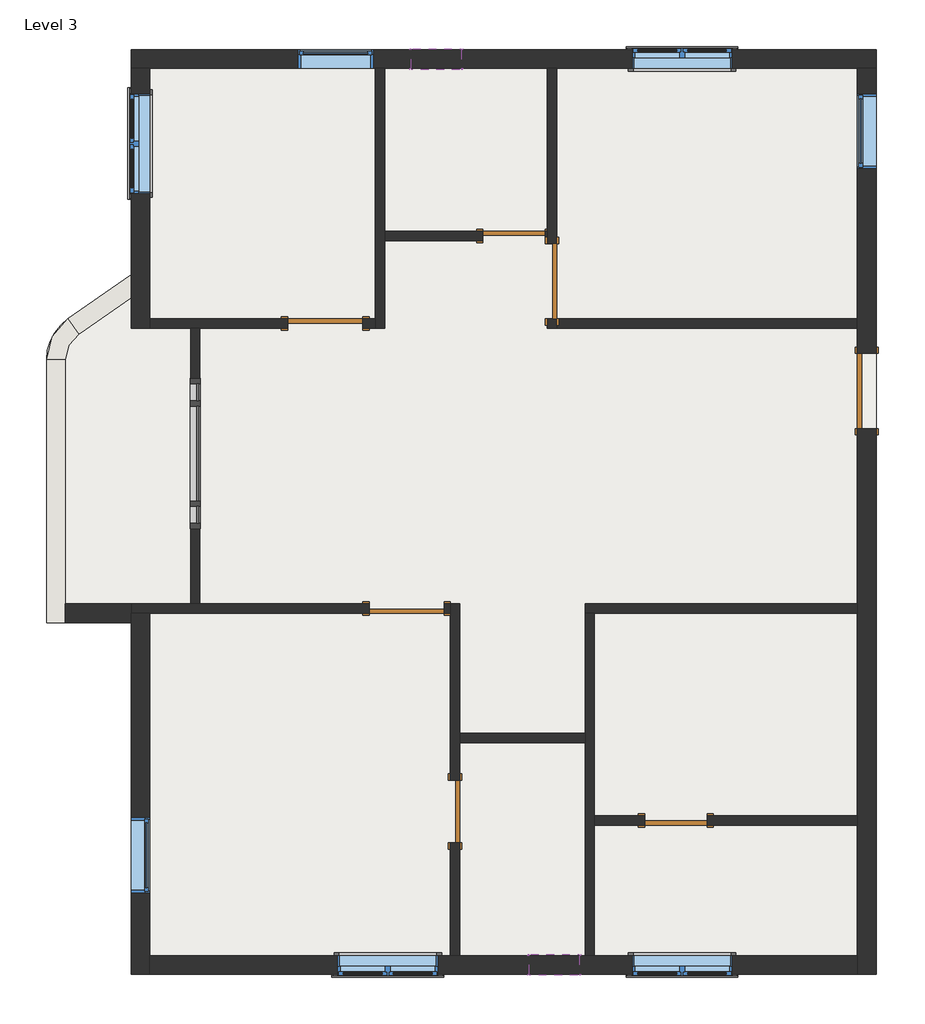
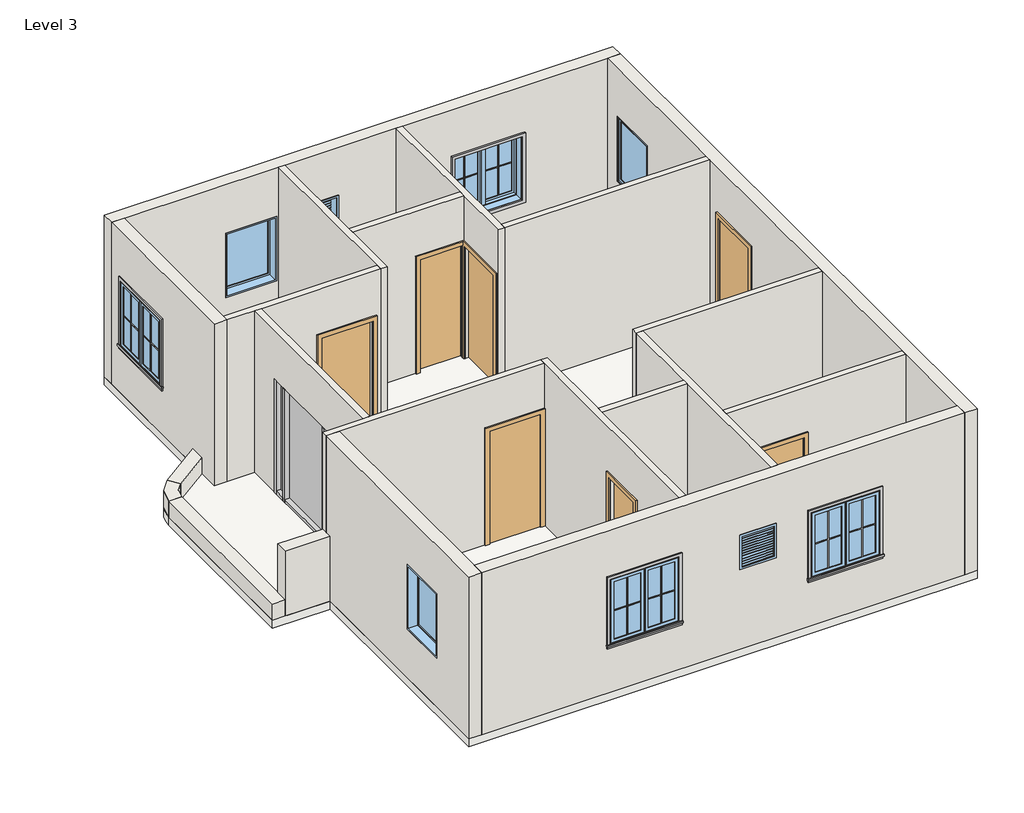
# One storey: 21 walls, 16 proxies, 9 windows, 7 doors, 7 members, 3 plates, 1 slab.
"""IFC4 building model written with IfcOpenShell, lengths in millimetres."""

from ifc_helpers import new_model, si_unit, point, frame, frame_2d, origin, place, context, project, spatial, polyline, circle_curve, trimmed, segment, composite_curve, outline, extrude, faceted_brep, transform, mapped, element, save
from components import muntin_pattern_2x2_muntin_pattern_2x2_4dfeb3f3, muntin_pattern_2x2_muntin_pattern_2x2_e852a7e4, trim_window_exterior_flat_with_sill_7cfdd449, trim_window_interior_flat_picture_frame_f1e0b15b, door_214872d5, door_78caadf7, door_e5f9f3c4, door_305aa2a5, door_0ca8825f, member_420b45ef, member_d7472725, member_7cbddb58, member_3374d9b6, system_panel_glazed_b82c55cd, system_panel_glazed_76d7ee11, window_c1f32544, window_af3140d2, window_f2d8fef0

model = new_model("IFC4")

# Units and contexts
model_context = context("Model", 3, world=origin())
ifc_project = project(units=[si_unit("LENGTHUNIT", "METRE", prefix="MILLI")], contexts=[model_context])

# Site, building, storey
site = spatial("IfcSite", under=ifc_project)
building = spatial("IfcBuilding", under=site)
storey = spatial("IfcBuildingStorey", under=building, Name="Level 3", Elevation=3200.4)

# Proxies
placement = place(None, origin())
muntin_pattern_2x2_muntin_pattern_2x2_shape = muntin_pattern_2x2_muntin_pattern_2x2_4dfeb3f3(model_context)
element("IfcBuildingElementProxy", 1, Name="Muntin Pattern_2x2 : Muntin Pattern_2x2", ObjectType="Muntin Pattern_2x2 : Muntin Pattern_2x2", at=placement, inside=storey, context=model_context, shape_type="MappedRepresentation", body=[
    mapped(muntin_pattern_2x2_muntin_pattern_2x2_shape, transform((-15529.7981107, 3990.1340181, 4184.65), x_axis=(0.0, 1.0, 0.0), y_axis=(-1.0, 0.0, 0.0), z_axis=(0.0, 0.0, 1.0))),
])
element("IfcBuildingElementProxy", 2, Name="Muntin Pattern_2x2 : Muntin Pattern_2x2", ObjectType="Muntin Pattern_2x2 : Muntin Pattern_2x2", at=placement, inside=storey, context=model_context, shape_type="MappedRepresentation", body=[
    mapped(muntin_pattern_2x2_muntin_pattern_2x2_shape, transform((-9136.9356107, 5426.8215181, 4184.65), x_axis=(1.0, 0.0, 0.0), y_axis=(0.0, 1.0, 0.0), z_axis=(0.0, 0.0, 1.0))),
])
element("IfcBuildingElementProxy", 3, Name="Muntin Pattern_2x2 : Muntin Pattern_2x2", ObjectType="Muntin Pattern_2x2 : Muntin Pattern_2x2", at=placement, inside=storey, context=model_context, shape_type="MappedRepresentation", body=[
    mapped(muntin_pattern_2x2_muntin_pattern_2x2_shape, transform((-12111.9106107, -5806.3284819, 4184.65), x_axis=(-1.0, 0.0, 0.0), y_axis=(0.0, -1.0, 0.0), z_axis=(0.0, 0.0, 1.0))),
])
element("IfcBuildingElementProxy", 4, Name="Muntin Pattern_2x2 : Muntin Pattern_2x2", ObjectType="Muntin Pattern_2x2 : Muntin Pattern_2x2", at=placement, inside=storey, context=model_context, shape_type="MappedRepresentation", body=[
    mapped(muntin_pattern_2x2_muntin_pattern_2x2_shape, transform((-8530.5106107, -5806.3284819, 4184.65), x_axis=(-1.0, 0.0, 0.0), y_axis=(0.0, -1.0, 0.0), z_axis=(0.0, 0.0, 1.0))),
])
muntin_pattern_2x2_muntin_pattern_2x2_2_shape = muntin_pattern_2x2_muntin_pattern_2x2_e852a7e4(model_context)
element("IfcBuildingElementProxy", 5, Name="Muntin Pattern_2x2 : Muntin Pattern_2x2", ObjectType="Muntin Pattern_2x2 : Muntin Pattern_2x2", at=placement, inside=storey, context=model_context, shape_type="MappedRepresentation", body=[
    mapped(muntin_pattern_2x2_muntin_pattern_2x2_2_shape, transform((-15529.7981107, 4596.5590181, 4184.65), x_axis=(0.0, -1.0, 0.0), y_axis=(1.0, 0.0, 0.0), z_axis=(0.0, 0.0, 1.0))),
])
element("IfcBuildingElementProxy", 6, Name="Muntin Pattern_2x2 : Muntin Pattern_2x2", ObjectType="Muntin Pattern_2x2 : Muntin Pattern_2x2", at=placement, inside=storey, context=model_context, shape_type="MappedRepresentation", body=[
    mapped(muntin_pattern_2x2_muntin_pattern_2x2_2_shape, transform((-8530.5106107, 5426.8215181, 4184.65), x_axis=(-1.0, 0.0, 0.0), y_axis=(0.0, -1.0, 0.0), z_axis=(0.0, 0.0, 1.0))),
])
element("IfcBuildingElementProxy", 7, Name="Muntin Pattern_2x2 : Muntin Pattern_2x2", ObjectType="Muntin Pattern_2x2 : Muntin Pattern_2x2", at=placement, inside=storey, context=model_context, shape_type="MappedRepresentation", body=[
    mapped(muntin_pattern_2x2_muntin_pattern_2x2_2_shape, transform((-12718.3356107, -5806.3284819, 4184.65), x_axis=(1.0, 0.0, 0.0), y_axis=(0.0, 1.0, 0.0), z_axis=(0.0, 0.0, 1.0))),
])
element("IfcBuildingElementProxy", 8, Name="Muntin Pattern_2x2 : Muntin Pattern_2x2", ObjectType="Muntin Pattern_2x2 : Muntin Pattern_2x2", at=placement, inside=storey, context=model_context, shape_type="MappedRepresentation", body=[
    mapped(muntin_pattern_2x2_muntin_pattern_2x2_2_shape, transform((-9136.9356107, -5806.3284819, 4184.65), x_axis=(1.0, 0.0, 0.0), y_axis=(0.0, 1.0, 0.0), z_axis=(0.0, 0.0, 1.0))),
])
trim_window_exterior_flat_with_sill_shape = trim_window_exterior_flat_with_sill_7cfdd449(model_context)
element("IfcBuildingElementProxy", 9, Name="Trim-Window-Exterior-Flat : with Sill", ObjectType="Trim-Window-Exterior-Flat : with Sill", at=placement, inside=storey, context=model_context, shape_type="MappedRepresentation", body=[
    mapped(trim_window_exterior_flat_with_sill_shape, transform((-15539.3231107, 4293.3465181, 5334.0), x_axis=(0.0, -1.0, 0.0), y_axis=(0.0, 0.0, 1.0), z_axis=(-1.0, 0.0, 0.0))),
])
element("IfcBuildingElementProxy", 10, Name="Trim-Window-Exterior-Flat : with Sill", ObjectType="Trim-Window-Exterior-Flat : with Sill", at=placement, inside=storey, context=model_context, shape_type="MappedRepresentation", body=[
    mapped(trim_window_exterior_flat_with_sill_shape, transform((-8833.7231107, 5436.3465181, 5334.0), x_axis=(-1.0, 0.0, 0.0), y_axis=(0.0, 0.0, 1.0), z_axis=(0.0, 1.0, 0.0))),
])
element("IfcBuildingElementProxy", 11, Name="Trim-Window-Exterior-Flat : with Sill", ObjectType="Trim-Window-Exterior-Flat : with Sill", at=placement, inside=storey, context=model_context, shape_type="MappedRepresentation", body=[
    mapped(trim_window_exterior_flat_with_sill_shape, transform((-12415.1231107, -5815.8534819, 5334.0), x_axis=(1.0, 0.0, 0.0), y_axis=(0.0, 0.0, 1.0), z_axis=(0.0, -1.0, 0.0))),
])
element("IfcBuildingElementProxy", 12, Name="Trim-Window-Exterior-Flat : with Sill", ObjectType="Trim-Window-Exterior-Flat : with Sill", at=placement, inside=storey, context=model_context, shape_type="MappedRepresentation", body=[
    mapped(trim_window_exterior_flat_with_sill_shape, transform((-8833.7231107, -5815.8534819, 5334.0), x_axis=(1.0, 0.0, 0.0), y_axis=(0.0, 0.0, 1.0), z_axis=(0.0, -1.0, 0.0))),
])
trim_window_interior_flat_picture_frame_shape = trim_window_interior_flat_picture_frame_f1e0b15b(model_context)
element("IfcBuildingElementProxy", 13, Name="Trim-Window-Interior-Flat : Picture Frame", ObjectType="Trim-Window-Interior-Flat : Picture Frame", at=placement, inside=storey, context=model_context, shape_type="MappedRepresentation", body=[
    mapped(trim_window_interior_flat_picture_frame_shape, transform((-15310.7231107, 4293.3465181, 5334.0), x_axis=(0.0, 1.0, 0.0), y_axis=(0.0, 0.0, 1.0), z_axis=(1.0, 0.0, 0.0))),
])
element("IfcBuildingElementProxy", 14, Name="Trim-Window-Interior-Flat : Picture Frame", ObjectType="Trim-Window-Interior-Flat : Picture Frame", at=placement, inside=storey, context=model_context, shape_type="MappedRepresentation", body=[
    mapped(trim_window_interior_flat_picture_frame_shape, transform((-8833.7231107, 5207.7465181, 5334.0), x_axis=(1.0, 0.0, 0.0), y_axis=(0.0, 0.0, 1.0), z_axis=(0.0, -1.0, 0.0))),
])
element("IfcBuildingElementProxy", 15, Name="Trim-Window-Interior-Flat : Picture Frame", ObjectType="Trim-Window-Interior-Flat : Picture Frame", at=placement, inside=storey, context=model_context, shape_type="MappedRepresentation", body=[
    mapped(trim_window_interior_flat_picture_frame_shape, transform((-12415.1231107, -5587.2534819, 5334.0), x_axis=(-1.0, 0.0, 0.0), y_axis=(0.0, 0.0, 1.0), z_axis=(0.0, 1.0, 0.0))),
])
element("IfcBuildingElementProxy", 16, Name="Trim-Window-Interior-Flat : Picture Frame", ObjectType="Trim-Window-Interior-Flat : Picture Frame", at=placement, inside=storey, context=model_context, shape_type="MappedRepresentation", body=[
    mapped(trim_window_interior_flat_picture_frame_shape, transform((-8833.7231107, -5587.2534819, 5334.0), x_axis=(-1.0, 0.0, 0.0), y_axis=(0.0, 0.0, 1.0), z_axis=(0.0, 1.0, 0.0))),
])

# Doors
door_shape = door_214872d5(model_context)
element("IfcDoor", 17, ObjectType="Single-Flush : 2'6\" X 7'", at=placement, inside=storey, context=model_context, shape_type="MappedRepresentation", body=[
    mapped(door_shape, transform((-10878.4231107, 3169.3965181, 3200.4), x_axis=(1.0, 0.0, 0.0), y_axis=(0.0, 1.0, 0.0), z_axis=(0.0, 0.0, 1.0))),
])
element("IfcDoor", 18, ObjectType="Single-Flush : 2'6\" X 7'", at=placement, inside=storey, context=model_context, shape_type="MappedRepresentation", body=[
    mapped(door_shape, transform((-8909.9231107, -3942.6034819, 3200.4), x_axis=(-1.0, 0.0, 0.0), y_axis=(0.0, -1.0, 0.0), z_axis=(0.0, 0.0, 1.0))),
])
door_2_shape = door_78caadf7(model_context)
element("IfcDoor", 19, ObjectType="Single-Flush : 2'6\" X 7'", at=placement, inside=storey, context=model_context, shape_type="MappedRepresentation", body=[
    mapped(door_2_shape, transform((-11595.9731107, -3834.6534819, 3200.4), x_axis=(0.0, 1.0, 0.0), y_axis=(-1.0, 0.0, 0.0), z_axis=(0.0, 0.0, 1.0))),
])
door_3_shape = door_e5f9f3c4(model_context)
element("IfcDoor", 20, ObjectType="Single-Flush : 36\" x 84\"", at=placement, inside=storey, context=model_context, shape_type="MappedRepresentation", body=[
    mapped(door_3_shape, transform((-13177.1231107, 2102.5965181, 3200.4), x_axis=(1.0, 0.0, 0.0), y_axis=(0.0, 1.0, 0.0), z_axis=(0.0, 0.0, 1.0))),
])
element("IfcDoor", 21, ObjectType="Single-Flush : 36\" x 84\"", at=placement, inside=storey, context=model_context, shape_type="MappedRepresentation", body=[
    mapped(door_3_shape, transform((-10414.8731107, 2618.6439204, 3200.4), x_axis=(0.0, -1.0, 0.0), y_axis=(1.0, 0.0, 0.0), z_axis=(0.0, 0.0, 1.0))),
])
door_4_shape = door_305aa2a5(model_context)
element("IfcDoor", 22, ObjectType="Single-Flush : 36\" x 84\"", at=placement, inside=storey, context=model_context, shape_type="MappedRepresentation", body=[
    mapped(door_4_shape, transform((-12186.5231107, -1364.5034819, 3200.4), x_axis=(1.0, 0.0, 0.0), y_axis=(0.0, 1.0, 0.0), z_axis=(0.0, 0.0, 1.0))),
])
door_5_shape = door_0ca8825f(model_context)
element("IfcDoor", 23, ObjectType="Single-Flush : 36\" x 84\"", at=placement, inside=storey, context=model_context, shape_type="MappedRepresentation", body=[
    mapped(door_5_shape, transform((-6585.8231107, 1283.4465181, 3200.4), x_axis=(0.0, 1.0, 0.0), y_axis=(-1.0, 0.0, 0.0), z_axis=(0.0, 0.0, 1.0))),
])

# Members
member_shape = member_420b45ef(model_context)
element("IfcMember", 24, ObjectType="Rectangular Mullion : 2.5\" x 5\" rectangular", at=placement, inside=storey, context=model_context, shape_type="MappedRepresentation", body=[
    mapped(member_shape, transform((-14758.2731107, 1372.3465181, 3200.4), x_axis=(0.0, 0.0, -1.0), y_axis=(-1.0, 0.0, 0.0), z_axis=(0.0, 1.0, 0.0))),
])
element("IfcMember", 25, ObjectType="Rectangular Mullion : 2.5\" x 5\" rectangular", at=placement, inside=storey, context=model_context, shape_type="MappedRepresentation", body=[
    mapped(member_shape, transform((-14758.2731107, -119.9034819, 3200.4), x_axis=(0.0, 0.0, -1.0), y_axis=(-1.0, 0.0, 0.0), z_axis=(0.0, 1.0, 0.0))),
])
member_2_shape = member_d7472725(model_context)
element("IfcMember", 26, ObjectType="Rectangular Mullion : 2.5\" x 5\" rectangular", at=placement, inside=storey, context=model_context, shape_type="MappedRepresentation", body=[
    mapped(member_2_shape, transform((-14758.2731107, 1099.2965181, 3200.4), x_axis=(0.0, 0.0, -1.0), y_axis=(-1.0, 0.0, 0.0), z_axis=(0.0, 1.0, 0.0))),
])
member_3_shape = member_7cbddb58(model_context)
element("IfcMember", 27, ObjectType="Rectangular Mullion : 2.5\" x 5\" rectangular", at=placement, inside=storey, context=model_context, shape_type="MappedRepresentation", body=[
    mapped(member_3_shape, transform((-14758.2731107, 1131.0465181, 3200.4), x_axis=(0.0, -1.0, 0.0), y_axis=(-1.0, 0.0, 0.0), z_axis=(0.0, 0.0, -1.0))),
])
element("IfcMember", 28, ObjectType="Rectangular Mullion : 2.5\" x 5\" rectangular", at=placement, inside=storey, context=model_context, shape_type="MappedRepresentation", body=[
    mapped(member_3_shape, transform((-14758.2731107, -88.1534819, 3200.4), x_axis=(0.0, -1.0, 0.0), y_axis=(-1.0, 0.0, 0.0), z_axis=(0.0, 0.0, -1.0))),
])
member_4_shape = member_3374d9b6(model_context)
element("IfcMember", 29, ObjectType="Rectangular Mullion : 2.5\" x 5\" rectangular", at=placement, inside=storey, context=model_context, shape_type="MappedRepresentation", body=[
    mapped(member_4_shape, transform((-14758.2731107, 1435.8465181, 5334.0), x_axis=(0.0, 1.0, 0.0), y_axis=(-1.0, 0.0, 0.0), z_axis=(0.0, 0.0, 1.0))),
])
element("IfcMember", 30, ObjectType="Rectangular Mullion : 2.5\" x 5\" rectangular", at=placement, inside=storey, context=model_context, shape_type="MappedRepresentation", body=[
    mapped(member_4_shape, transform((-14758.2731107, -392.9534819, 3200.4), x_axis=(0.0, -1.0, 0.0), y_axis=(-1.0, 0.0, 0.0), z_axis=(0.0, 0.0, -1.0))),
])

# Plates
system_panel_glazed_shape = system_panel_glazed_b82c55cd(model_context)
element("IfcPlate", 31, ObjectType="System Panel : Glazed", at=placement, inside=storey, context=model_context, shape_type="MappedRepresentation", body=[
    mapped(system_panel_glazed_shape, transform((-14758.2731107, 1267.5715181, 3263.9), x_axis=(0.0, -1.0, 0.0), y_axis=(1.0, 0.0, 0.0), z_axis=(0.0, 0.0, 1.0))),
])
element("IfcPlate", 32, ObjectType="System Panel : Glazed", at=placement, inside=storey, context=model_context, shape_type="MappedRepresentation", body=[
    mapped(system_panel_glazed_shape, transform((-14758.2731107, -224.6784819, 3263.9), x_axis=(0.0, -1.0, 0.0), y_axis=(1.0, 0.0, 0.0), z_axis=(0.0, 0.0, 1.0))),
])
system_panel_glazed_2_shape = system_panel_glazed_76d7ee11(model_context)
element("IfcPlate", 33, ObjectType="System Panel : Glazed", at=placement, inside=storey, context=model_context, shape_type="MappedRepresentation", body=[
    mapped(system_panel_glazed_2_shape, transform((-14758.2731107, 521.4465181, 3263.9), x_axis=(0.0, -1.0, 0.0), y_axis=(1.0, 0.0, 0.0), z_axis=(0.0, 0.0, 1.0))),
])

# Slab
element("IfcSlab", 34, ObjectType="6\"", at=placement, inside=storey, context=model_context, shape_type="SweptSolid", body=[
    extrude(outline(composite_curve([segment(polyline([(-6471.5231107, 5436.3465181), (-6471.5231107, -5815.8534819), (-15539.3231107, -5815.8534819), (-15539.3231107, -1535.9534819), (-16568.0231107, -1535.9534819), (-16568.0231107, 1661.5585867)]), True, "CONTINUOUS"), segment(trimmed(circle_curve(frame_2d((-15958.4231107, 1661.5585867)), 609.6), [point((-16568.0231107, 1661.5585867))], [point((-16308.0753063, 2160.9136729))], False, "CARTESIAN"), True, "CONTINUOUS"), segment(polyline([(-16308.0753063, 2160.9136729), (-15539.3231107, 2699.1997553), (-15539.3231107, 5436.3465181), (-6471.5231107, 5436.3465181)]), True, "CONTINUOUS")], self_intersect=False)), frame((0.0, 0.0, 3048.0), z_axis=(0.0, 0.0, 1.0), x_axis=(1.0, 0.0, 0.0)), (0.0, 0.0, 1.0), 152.4),
])

# Walls
element("IfcWall", 35, ObjectType="4.5\"", at=placement, inside=storey, context=model_context, shape_type="Brep", body=[
    faceted_brep([(-12567.5231107, 5207.7465181, 3200.4), (-12567.5231107, 2159.7465181, 3200.4), (-12567.5231107, 2045.4465181, 3200.4), (-12567.5231107, 2045.4465181, 6248.4), (-12567.5231107, 2159.7465181, 6248.4), (-12567.5231107, 5207.7465181, 6248.4), (-12453.2231107, 5207.7465181, 3200.4), (-12453.2231107, 5207.7465181, 6248.4), (-12453.2231107, 3226.5465181, 6248.4), (-12453.2231107, 3112.2465181, 6248.4), (-12453.2231107, 2045.4465181, 6248.4), (-12453.2231107, 2045.4465181, 3200.4), (-12453.2231107, 3112.2465181, 3200.4), (-12453.2231107, 3226.5465181, 3200.4)], [[[0, 1, 2, 3, 4, 5]], [[6, 7, 8, 9, 10, 11, 12, 13]], [[2, 1, 0, 6, 13, 12, 11]], [[5, 4, 3, 10, 9, 8, 7]], [[0, 5, 7, 6]], [[3, 2, 11, 10]]]),
])
element("IfcWall", 36, ObjectType="4.5\"", at=placement, inside=storey, context=model_context, shape_type="Brep", body=[
    faceted_brep([(-12719.9231107, 2045.4465181, 5334.0), (-12719.9231107, 2045.4465181, 3200.4), (-12567.5231107, 2045.4465181, 3200.4), (-12567.5231107, 2045.4465181, 6248.4), (-14701.1231107, 2045.4465181, 6248.4), (-14815.4231107, 2045.4465181, 6248.4), (-15310.7231107, 2045.4465181, 6248.4), (-15310.7231107, 2045.4465181, 3200.4), (-14815.4231107, 2045.4465181, 3200.4), (-14701.1231107, 2045.4465181, 3200.4), (-13634.3231107, 2045.4465181, 3200.4), (-13634.3231107, 2045.4465181, 5334.0), (-12567.5231107, 2159.7465181, 3200.4), (-12719.9231107, 2159.7465181, 3200.4), (-12719.9231107, 2159.7465181, 5334.0), (-13634.3231107, 2159.7465181, 5334.0), (-13634.3231107, 2159.7465181, 3200.4), (-15310.7231107, 2159.7465181, 3200.4), (-15310.7231107, 2159.7465181, 6248.4), (-12567.5231107, 2159.7465181, 6248.4)], [[[0, 1, 2, 3, 4, 5, 6, 7, 8, 9, 10, 11]], [[12, 13, 14, 15, 16, 17, 18, 19]], [[2, 1, 13, 12]], [[10, 9, 8, 7, 17, 16]], [[6, 5, 4, 3, 19, 18]], [[3, 2, 12, 19]], [[7, 6, 18, 17]], [[14, 13, 1, 0]], [[15, 14, 0, 11]], [[16, 15, 11, 10]]]),
])
element("IfcWall", 37, ObjectType="4.5\"", at=placement, inside=storey, context=model_context, shape_type="Brep", body=[
    faceted_brep([(-10472.0231107, 2161.4439204, 5334.0), (-10472.0231107, 2161.4439204, 3200.4), (-10472.0231107, 2045.4465181, 3200.4), (-10472.0231107, 2045.4465181, 6248.4), (-10472.0231107, 3112.2465181, 6248.4), (-10472.0231107, 3226.5465181, 6248.4), (-10472.0231107, 5207.7465181, 6248.4), (-10472.0231107, 5207.7465181, 3200.4), (-10472.0231107, 3226.5465181, 3200.4), (-10472.0231107, 3112.2465181, 3200.4), (-10472.0231107, 3075.8439204, 3200.4), (-10472.0231107, 3075.8439204, 5334.0), (-10357.7231107, 2045.4465181, 3200.4), (-10357.7231107, 2159.7465181, 3200.4), (-10357.7231107, 2161.4439204, 3200.4), (-10357.7231107, 2161.4439204, 5334.0), (-10357.7231107, 3075.8439204, 5334.0), (-10357.7231107, 3075.8439204, 3200.4), (-10357.7231107, 5207.7465181, 3200.4), (-10357.7231107, 5207.7465181, 6248.4), (-10357.7231107, 2159.7465181, 6248.4), (-10357.7231107, 2045.4465181, 6248.4)], [[[0, 1, 2, 3, 4, 5, 6, 7, 8, 9, 10, 11]], [[12, 13, 14, 15, 16, 17, 18, 19, 20, 21]], [[2, 1, 14, 13, 12]], [[10, 9, 8, 7, 18, 17]], [[6, 5, 4, 3, 21, 20, 19]], [[7, 6, 19, 18]], [[3, 2, 12, 21]], [[15, 14, 1, 0]], [[16, 15, 0, 11]], [[17, 16, 11, 10]]]),
])
element("IfcWall", 38, ObjectType="4.5\"", at=placement, inside=storey, context=model_context, shape_type="SweptSolid", body=[
    extrude(outline(polyline([(5334.0, -10497.4231107), (3200.4, -10497.4231107), (3200.4, -10472.0231107), (6248.4, -10472.0231107), (6248.4, -12453.2231107), (3200.4, -12453.2231107), (3200.4, -11259.4231107), (5334.0, -11259.4231107), (5334.0, -10497.4231107)])), frame((0.0, 3112.2465181, 0.0), z_axis=(0.0, 1.0, 0.0), x_axis=(0.0, 0.0, 1.0)), (0.0, 0.0, 1.0), 114.3),
])
element("IfcWall", 39, ObjectType="4.5\"", at=placement, inside=storey, context=model_context, shape_type="SweptSolid", body=[
    extrude(outline(polyline([(-10357.7231107, 2159.7465181), (-6700.1231107, 2159.7465181), (-6700.1231107, 2045.4465181), (-10357.7231107, 2045.4465181), (-10357.7231107, 2159.7465181)])), frame((0.0, 0.0, 3200.4), z_axis=(0.0, 0.0, 1.0), x_axis=(1.0, 0.0, 0.0)), (0.0, 0.0, 1.0), 3048.0),
])
element("IfcWall", 40, ObjectType="4.5\"", at=placement, inside=storey, context=model_context, shape_type="Brep", body=[
    faceted_brep([(-6700.1231107, -1307.3534819, 3200.4), (-10014.8231107, -1307.3534819, 3200.4), (-10014.8231107, -1307.3534819, 6248.4), (-6700.1231107, -1307.3534819, 6248.4), (-6700.1231107, -1421.6534819, 3200.4), (-6700.1231107, -1421.6534819, 6248.4), (-9900.5231107, -1421.6534819, 6248.4), (-10014.8231107, -1421.6534819, 6248.4), (-10014.8231107, -1421.6534819, 3200.4), (-9900.5231107, -1421.6534819, 3200.4)], [[[0, 1, 2, 3]], [[4, 5, 6, 7, 8, 9]], [[1, 0, 4, 9, 8]], [[3, 2, 7, 6, 5]], [[0, 3, 5, 4]], [[2, 1, 8, 7]]]),
])
element("IfcWall", 41, ObjectType="4.5\"", at=placement, inside=storey, context=model_context, shape_type="SweptSolid", body=[
    extrude(outline(polyline([(3200.4, -9900.5231107), (3200.4, -9290.9231107), (5334.0, -9290.9231107), (5334.0, -8528.9231107), (3200.4, -8528.9231107), (3200.4, -6700.1231107), (6248.4, -6700.1231107), (6248.4, -9900.5231107), (3200.4, -9900.5231107)])), frame((0.0, -3999.7534819, 0.0), z_axis=(0.0, 1.0, 0.0), x_axis=(0.0, 0.0, 1.0)), (0.0, 0.0, 1.0), 114.3),
])
element("IfcWall", 42, ObjectType="4.5\"", at=placement, inside=storey, context=model_context, shape_type="Brep", body=[
    faceted_brep([(-9900.5231107, -5587.2534819, 3200.4), (-9900.5231107, -3999.7534819, 3200.4), (-9900.5231107, -3885.4534819, 3200.4), (-9900.5231107, -1421.6534819, 3200.4), (-9900.5231107, -1421.6534819, 6248.4), (-9900.5231107, -3885.4534819, 6248.4), (-9900.5231107, -3999.7534819, 6248.4), (-9900.5231107, -5587.2534819, 6248.4), (-10014.8231107, -5587.2534819, 3200.4), (-10014.8231107, -5587.2534819, 6248.4), (-10014.8231107, -2996.4534819, 6248.4), (-10014.8231107, -2882.1534819, 6248.4), (-10014.8231107, -1421.6534819, 6248.4), (-10014.8231107, -1421.6534819, 3200.4), (-10014.8231107, -2882.1534819, 3200.4), (-10014.8231107, -2996.4534819, 3200.4)], [[[0, 1, 2, 3, 4, 5, 6, 7]], [[8, 9, 10, 11, 12, 13, 14, 15]], [[3, 2, 1, 0, 8, 15, 14, 13]], [[7, 6, 5, 4, 12, 11, 10, 9]], [[0, 7, 9, 8]], [[4, 3, 13, 12]]]),
])
element("IfcWall", 43, ObjectType="4.5\"", at=placement, inside=storey, context=model_context, shape_type="Brep", body=[
    faceted_brep([(-11538.8231107, -3453.6534819, 5334.0), (-11538.8231107, -3453.6534819, 3200.4), (-11538.8231107, -2996.4534819, 3200.4), (-11538.8231107, -2882.1534819, 3200.4), (-11538.8231107, -1307.3534819, 3200.4), (-11538.8231107, -1307.3534819, 6248.4), (-11538.8231107, -2882.1534819, 6248.4), (-11538.8231107, -2996.4534819, 6248.4), (-11538.8231107, -5587.2534819, 6248.4), (-11538.8231107, -5587.2534819, 3200.4), (-11538.8231107, -4215.6534819, 3200.4), (-11538.8231107, -4215.6534819, 5334.0), (-11653.1231107, -1307.3534819, 3200.4), (-11653.1231107, -1421.6534819, 3200.4), (-11653.1231107, -3453.6534819, 3200.4), (-11653.1231107, -3453.6534819, 5334.0), (-11653.1231107, -4215.6534819, 5334.0), (-11653.1231107, -4215.6534819, 3200.4), (-11653.1231107, -5587.2534819, 3200.4), (-11653.1231107, -5587.2534819, 6248.4), (-11653.1231107, -1421.6534819, 6248.4), (-11653.1231107, -1307.3534819, 6248.4)], [[[0, 1, 2, 3, 4, 5, 6, 7, 8, 9, 10, 11]], [[12, 13, 14, 15, 16, 17, 18, 19, 20, 21]], [[10, 9, 18, 17]], [[4, 3, 2, 1, 14, 13, 12]], [[8, 7, 6, 5, 21, 20, 19]], [[9, 8, 19, 18]], [[5, 4, 12, 21]], [[15, 14, 1, 0]], [[16, 15, 0, 11]], [[17, 16, 11, 10]]]),
])
element("IfcWall", 44, ObjectType="4.5\"", at=placement, inside=storey, context=model_context, shape_type="SweptSolid", body=[
    extrude(outline(polyline([(-10014.8231107, -2996.4534819), (-11538.8231107, -2996.4534819), (-11538.8231107, -2882.1534819), (-10014.8231107, -2882.1534819), (-10014.8231107, -2996.4534819)])), frame((0.0, 0.0, 3200.4), z_axis=(0.0, 0.0, 1.0), x_axis=(1.0, 0.0, 0.0)), (0.0, 0.0, 1.0), 3048.0),
])
element("IfcWall", 45, ObjectType="4.5\"", at=placement, inside=storey, context=model_context, shape_type="Brep", body=[
    faceted_brep([(-11653.1231107, -1307.3534819, 3200.4), (-11729.3231107, -1307.3534819, 3200.4), (-11729.3231107, -1307.3534819, 5334.0), (-12643.7231107, -1307.3534819, 5334.0), (-12643.7231107, -1307.3534819, 3200.4), (-14701.1231107, -1307.3534819, 3200.4), (-14815.4231107, -1307.3534819, 3200.4), (-15539.3231107, -1307.3534819, 3200.4), (-15539.3231107, -1307.3534819, 4419.6), (-15539.3231107, -1307.3534819, 6248.4), (-14815.4231107, -1307.3534819, 6248.4), (-14701.1231107, -1307.3534819, 6248.4), (-11653.1231107, -1307.3534819, 6248.4), (-11729.3231107, -1421.6534819, 5334.0), (-11729.3231107, -1421.6534819, 3200.4), (-11653.1231107, -1421.6534819, 3200.4), (-11653.1231107, -1421.6534819, 6248.4), (-15310.7231107, -1421.6534819, 6248.4), (-15539.3231107, -1421.6534819, 6248.4), (-15539.3231107, -1421.6534819, 3200.4), (-15310.7231107, -1421.6534819, 3200.4), (-12643.7231107, -1421.6534819, 3200.4), (-12643.7231107, -1421.6534819, 5334.0)], [[[0, 1, 2, 3, 4, 5, 6, 7, 8, 9, 10, 11, 12]], [[13, 14, 15, 16, 17, 18, 19, 20, 21, 22]], [[15, 14, 1, 0]], [[21, 20, 19, 7, 6, 5, 4]], [[12, 11, 10, 9, 18, 17, 16]], [[0, 12, 16, 15]], [[2, 1, 14, 13]], [[3, 2, 13, 22]], [[4, 3, 22, 21]], [[7, 19, 18, 9, 8]]]),
])
element("IfcWall", 46, ObjectType="4.5\"", at=placement, inside=storey, context=model_context, shape_type="SweptSolid", body=[
    extrude(outline(polyline([(-1307.3534819, 6248.4), (2045.4465181, 6248.4), (2045.4465181, 3200.4), (1435.8465181, 3200.4), (1435.8465181, 5334.0), (-392.9534819, 5334.0), (-392.9534819, 3200.4), (-1307.3534819, 3200.4), (-1307.3534819, 6248.4)])), frame((-14815.4231107, 0.0, 0.0), z_axis=(1.0, 0.0, 0.0), x_axis=(0.0, 1.0, 0.0)), (0.0, 0.0, 1.0), 114.3),
])
element("IfcWall", 47, ObjectType="9\"", at=placement, inside=storey, context=model_context, shape_type="Brep", body=[
    faceted_brep([(-15539.3231107, 5207.7465181, 3200.4), (-15310.7231107, 5207.7465181, 3200.4), (-12567.5231107, 5207.7465181, 3200.4), (-12453.2231107, 5207.7465181, 3200.4), (-10472.0231107, 5207.7465181, 3200.4), (-10357.7231107, 5207.7465181, 3200.4), (-6700.1231107, 5207.7465181, 3200.4), (-6471.5231107, 5207.7465181, 3200.4), (-6471.5231107, 5207.7465181, 6248.4), (-6700.1231107, 5207.7465181, 6248.4), (-10357.7231107, 5207.7465181, 6248.4), (-10472.0231107, 5207.7465181, 6248.4), (-12453.2231107, 5207.7465181, 6248.4), (-12567.5231107, 5207.7465181, 6248.4), (-15310.7231107, 5207.7465181, 6248.4), (-15539.3231107, 5207.7465181, 6248.4), (-12129.3731107, 5207.7465181, 5334.0), (-11519.7731107, 5207.7465181, 5334.0), (-11519.7731107, 5207.7465181, 4724.4), (-12129.3731107, 5207.7465181, 4724.4), (-8224.1231107, 5207.7465181, 5334.0), (-8224.1231107, 5207.7465181, 4114.8), (-9443.3231107, 5207.7465181, 4114.8), (-9443.3231107, 5207.7465181, 5334.0), (-12592.9231107, 5207.7465181, 5334.0), (-12592.9231107, 5207.7465181, 4114.8), (-13507.3231107, 5207.7465181, 4114.8), (-13507.3231107, 5207.7465181, 5334.0), (-15539.3231107, 5436.3465181, 3200.4), (-15539.3231107, 5436.3465181, 6248.4), (-6471.5231107, 5436.3465181, 6248.4), (-6471.5231107, 5436.3465181, 3200.4), (-12129.3731107, 5436.3465181, 5334.0), (-12129.3731107, 5436.3465181, 4724.4), (-11519.7731107, 5436.3465181, 4724.4), (-11519.7731107, 5436.3465181, 5334.0), (-8224.1231107, 5436.3465181, 5334.0), (-9443.3231107, 5436.3465181, 5334.0), (-9443.3231107, 5436.3465181, 4114.8), (-8224.1231107, 5436.3465181, 4114.8), (-12592.9231107, 5436.3465181, 5334.0), (-13507.3231107, 5436.3465181, 5334.0), (-13507.3231107, 5436.3465181, 4114.8), (-12592.9231107, 5436.3465181, 4114.8)], [[[0, 1, 2, 3, 4, 5, 6, 7, 8, 9, 10, 11, 12, 13, 14, 15], [16, 17, 18, 19], [20, 21, 22, 23], [24, 25, 26, 27]], [[28, 29, 30, 31], [32, 33, 34, 35], [36, 37, 38, 39], [40, 41, 42, 43]], [[7, 6, 5, 4, 3, 2, 1, 0, 28, 31]], [[15, 14, 13, 12, 11, 10, 9, 8, 30, 29]], [[0, 15, 29, 28]], [[8, 7, 31, 30]], [[33, 32, 16, 19]], [[34, 33, 19, 18]], [[35, 34, 18, 17]], [[32, 35, 17, 16]], [[21, 20, 36, 39]], [[22, 21, 39, 38]], [[23, 22, 38, 37]], [[20, 23, 37, 36]], [[25, 24, 40, 43]], [[26, 25, 43, 42]], [[27, 26, 42, 41]], [[24, 27, 41, 40]]]),
])
element("IfcWall", 48, ObjectType="9\"", at=placement, inside=storey, context=model_context, shape_type="Brep", body=[
    faceted_brep([(-15539.3231107, 5207.7465181, 3200.4), (-15539.3231107, 2699.1997553, 3200.4), (-15539.3231107, 2420.1306843, 3200.4), (-15539.3231107, 2045.4465181, 3200.4), (-15539.3231107, 2045.4465181, 6248.4), (-15539.3231107, 5207.7465181, 6248.4), (-15539.3231107, 4902.9465181, 5334.0), (-15539.3231107, 3683.7465181, 5334.0), (-15539.3231107, 3683.7465181, 4114.8), (-15539.3231107, 4902.9465181, 4114.8), (-15310.7231107, 5207.7465181, 3200.4), (-15310.7231107, 5207.7465181, 6248.4), (-15310.7231107, 2159.7465181, 6248.4), (-15310.7231107, 2045.4465181, 6248.4), (-15310.7231107, 2045.4465181, 3200.4), (-15310.7231107, 2159.7465181, 3200.4), (-15310.7231107, 4902.9465181, 5334.0), (-15310.7231107, 4902.9465181, 4114.8), (-15310.7231107, 3683.7465181, 4114.8), (-15310.7231107, 3683.7465181, 5334.0)], [[[0, 1, 2, 3, 4, 5], [6, 7, 8, 9]], [[10, 11, 12, 13, 14, 15], [16, 17, 18, 19]], [[3, 2, 1, 0, 10, 15, 14]], [[5, 4, 13, 12, 11]], [[0, 5, 11, 10]], [[4, 3, 14, 13]], [[17, 16, 6, 9]], [[18, 17, 9, 8]], [[19, 18, 8, 7]], [[16, 19, 7, 6]]]),
])
element("IfcWall", 49, ObjectType="9\"", at=placement, inside=storey, context=model_context, shape_type="Brep", body=[
    faceted_brep([(-6700.1231107, 5207.7465181, 3200.4), (-6700.1231107, 2159.7465181, 3200.4), (-6700.1231107, 2045.4465181, 3200.4), (-6700.1231107, 1740.6465181, 3200.4), (-6700.1231107, 1740.6465181, 5334.0), (-6700.1231107, 826.2465181, 5334.0), (-6700.1231107, 826.2465181, 3200.4), (-6700.1231107, -1307.3534819, 3200.4), (-6700.1231107, -1421.6534819, 3200.4), (-6700.1231107, -3885.4534819, 3200.4), (-6700.1231107, -3999.7534819, 3200.4), (-6700.1231107, -5587.2534819, 3200.4), (-6700.1231107, -5815.8534819, 3200.4), (-6700.1231107, -5815.8534819, 6248.4), (-6700.1231107, -5587.2534819, 6248.4), (-6700.1231107, -3999.7534819, 6248.4), (-6700.1231107, -3885.4534819, 6248.4), (-6700.1231107, -1421.6534819, 6248.4), (-6700.1231107, -1307.3534819, 6248.4), (-6700.1231107, 2045.4465181, 6248.4), (-6700.1231107, 2159.7465181, 6248.4), (-6700.1231107, 5207.7465181, 6248.4), (-6700.1231107, 4902.9465181, 5334.0), (-6700.1231107, 3988.5465181, 5334.0), (-6700.1231107, 3988.5465181, 4114.8), (-6700.1231107, 4902.9465181, 4114.8), (-6471.5231107, 1740.6465181, 5334.0), (-6471.5231107, 1740.6465181, 3200.4), (-6471.5231107, 5207.7465181, 3200.4), (-6471.5231107, 5207.7465181, 6248.4), (-6471.5231107, -5815.8534819, 6248.4), (-6471.5231107, -5815.8534819, 3200.4), (-6471.5231107, 826.2465181, 3200.4), (-6471.5231107, 826.2465181, 5334.0), (-6471.5231107, 4902.9465181, 5334.0), (-6471.5231107, 4902.9465181, 4114.8), (-6471.5231107, 3988.5465181, 4114.8), (-6471.5231107, 3988.5465181, 5334.0)], [[[0, 1, 2, 3, 4, 5, 6, 7, 8, 9, 10, 11, 12, 13, 14, 15, 16, 17, 18, 19, 20, 21], [22, 23, 24, 25]], [[26, 27, 28, 29, 30, 31, 32, 33], [34, 35, 36, 37]], [[32, 31, 12, 11, 10, 9, 8, 7, 6]], [[28, 27, 3, 2, 1, 0]], [[21, 20, 19, 18, 17, 16, 15, 14, 13, 30, 29]], [[0, 21, 29, 28]], [[13, 12, 31, 30]], [[35, 34, 22, 25]], [[36, 35, 25, 24]], [[37, 36, 24, 23]], [[34, 37, 23, 22]], [[4, 3, 27, 26]], [[5, 4, 26, 33]], [[6, 5, 33, 32]]]),
])
element("IfcWall", 50, ObjectType="9\"", at=placement, inside=storey, context=model_context, shape_type="Brep", body=[
    faceted_brep([(-15310.7231107, -5815.8534819, 3200.4), (-6700.1231107, -5815.8534819, 3200.4), (-6700.1231107, -5815.8534819, 6248.4), (-15310.7231107, -5815.8534819, 6248.4), (-10084.6731107, -5815.8534819, 5334.0), (-10084.6731107, -5815.8534819, 4724.4), (-10694.2731107, -5815.8534819, 4724.4), (-10694.2731107, -5815.8534819, 5334.0), (-13024.7231107, -5815.8534819, 5334.0), (-11805.5231107, -5815.8534819, 5334.0), (-11805.5231107, -5815.8534819, 4114.8), (-13024.7231107, -5815.8534819, 4114.8), (-9443.3231107, -5815.8534819, 5334.0), (-8224.1231107, -5815.8534819, 5334.0), (-8224.1231107, -5815.8534819, 4114.8), (-9443.3231107, -5815.8534819, 4114.8), (-15310.7231107, -5587.2534819, 3200.4), (-15310.7231107, -5587.2534819, 6248.4), (-11653.1231107, -5587.2534819, 6248.4), (-11538.8231107, -5587.2534819, 6248.4), (-10014.8231107, -5587.2534819, 6248.4), (-9900.5231107, -5587.2534819, 6248.4), (-6700.1231107, -5587.2534819, 6248.4), (-6700.1231107, -5587.2534819, 3200.4), (-9900.5231107, -5587.2534819, 3200.4), (-10014.8231107, -5587.2534819, 3200.4), (-11538.8231107, -5587.2534819, 3200.4), (-11653.1231107, -5587.2534819, 3200.4), (-10084.6731107, -5587.2534819, 5334.0), (-10694.2731107, -5587.2534819, 5334.0), (-10694.2731107, -5587.2534819, 4724.4), (-10084.6731107, -5587.2534819, 4724.4), (-13024.7231107, -5587.2534819, 5334.0), (-13024.7231107, -5587.2534819, 4114.8), (-11805.5231107, -5587.2534819, 4114.8), (-11805.5231107, -5587.2534819, 5334.0), (-9443.3231107, -5587.2534819, 5334.0), (-9443.3231107, -5587.2534819, 4114.8), (-8224.1231107, -5587.2534819, 4114.8), (-8224.1231107, -5587.2534819, 5334.0)], [[[0, 1, 2, 3], [4, 5, 6, 7], [8, 9, 10, 11], [12, 13, 14, 15]], [[16, 17, 18, 19, 20, 21, 22, 23, 24, 25, 26, 27], [28, 29, 30, 31], [32, 33, 34, 35], [36, 37, 38, 39]], [[1, 0, 16, 27, 26, 25, 24, 23]], [[3, 2, 22, 21, 20, 19, 18, 17]], [[0, 3, 17, 16]], [[2, 1, 23, 22]], [[5, 4, 28, 31]], [[6, 5, 31, 30]], [[7, 6, 30, 29]], [[4, 7, 29, 28]], [[33, 32, 8, 11]], [[34, 33, 11, 10]], [[35, 34, 10, 9]], [[32, 35, 9, 8]], [[37, 36, 12, 15]], [[38, 37, 15, 14]], [[39, 38, 14, 13]], [[36, 39, 13, 12]]]),
])
element("IfcWall", 51, ObjectType="9\"", at=placement, inside=storey, context=model_context, shape_type="Brep", body=[
    faceted_brep([(-15539.3231107, -1421.6534819, 6248.4), (-15539.3231107, -1421.6534819, 3200.4), (-15539.3231107, -1535.9534819, 3200.4), (-15539.3231107, -5815.8534819, 3200.4), (-15539.3231107, -5815.8534819, 6248.4), (-15539.3231107, -4825.2534819, 5334.0), (-15539.3231107, -4825.2534819, 4114.8), (-15539.3231107, -3910.8534819, 4114.8), (-15539.3231107, -3910.8534819, 5334.0), (-15310.7231107, -1421.6534819, 3200.4), (-15310.7231107, -1421.6534819, 6248.4), (-15310.7231107, -5587.2534819, 6248.4), (-15310.7231107, -5815.8534819, 6248.4), (-15310.7231107, -5815.8534819, 3200.4), (-15310.7231107, -5587.2534819, 3200.4), (-15310.7231107, -4825.2534819, 5334.0), (-15310.7231107, -3910.8534819, 5334.0), (-15310.7231107, -3910.8534819, 4114.8), (-15310.7231107, -4825.2534819, 4114.8)], [[[0, 1, 2, 3, 4], [5, 6, 7, 8]], [[9, 10, 11, 12, 13, 14], [15, 16, 17, 18]], [[3, 2, 1, 9, 14, 13]], [[0, 4, 12, 11, 10]], [[4, 3, 13, 12]], [[0, 10, 9, 1]], [[6, 5, 15, 18]], [[7, 6, 18, 17]], [[8, 7, 17, 16]], [[5, 8, 16, 15]]]),
])
element("IfcWall", 52, ObjectType="9\"", at=placement, inside=storey, context=model_context, shape_type="Brep", body=[
    faceted_brep([(-16339.4231107, -1535.9534819, 3200.4), (-16339.4231107, -1307.3534819, 3200.4), (-16339.4231107, 1661.5585867, 3200.4), (-16339.4231107, 1661.5585867, 3505.2), (-16339.4231107, -1535.9534819, 3505.2), (-16568.0231107, -1535.9534819, 3200.4), (-16568.0231107, -1535.9534819, 3505.2), (-16568.0231107, 1661.5585867, 3505.2), (-16568.0231107, 1661.5585867, 3200.4)], [[[0, 1, 2, 3, 4]], [[5, 6, 7, 8]], [[2, 1, 0, 5, 8]], [[3, 2, 8, 7]], [[4, 3, 7, 6]], [[0, 4, 6, 5]]]),
])
element("IfcWall", 53, ObjectType="9\"", at=placement, inside=storey, context=model_context, shape_type="Brep", body=[
    faceted_brep([(-15539.3231107, -1307.3534819, 3200.4), (-16339.4231107, -1307.3534819, 3200.4), (-16339.4231107, -1307.3534819, 4419.6), (-15539.3231107, -1307.3534819, 4419.6), (-15539.3231107, -1535.9534819, 3200.4), (-15539.3231107, -1535.9534819, 4419.6), (-16339.4231107, -1535.9534819, 4419.6), (-16339.4231107, -1535.9534819, 3505.2), (-16339.4231107, -1535.9534819, 3200.4), (-15539.3231107, -1421.6534819, 3200.4)], [[[0, 1, 2, 3]], [[4, 5, 6, 7, 8]], [[1, 0, 9, 4, 8]], [[3, 2, 6, 5]], [[0, 3, 5, 4, 9]], [[2, 1, 8, 7, 6]]]),
])
element("IfcWall", 54, ObjectType="9\"", at=placement, inside=storey, context=model_context, shape_type="SweptSolid", body=[
    extrude(outline(polyline([(-15539.3231107, 2420.1306843), (-16176.9557329, 1973.6555156), (-16308.0753063, 2160.9136729), (-15539.3231107, 2699.1997553), (-15539.3231107, 2420.1306843)])), frame((0.0, 0.0, 3200.4), z_axis=(0.0, 0.0, 1.0), x_axis=(1.0, 0.0, 0.0)), (0.0, 0.0, 1.0), 304.8),
])
element("IfcWall", 55, ObjectType="9\"", at=placement, inside=storey, context=model_context, shape_type="SweptSolid", body=[
    extrude(outline(composite_curve([segment(polyline([(-16308.0753063, 2160.9136729), (-16176.9557329, 1973.6555156)]), True, "CONTINUOUS"), segment(trimmed(circle_curve(frame_2d((-15958.4231107, 1661.5585867)), 381.0), [point((-16176.9557329, 1973.6555156))], [point((-16339.4231107, 1661.5585867))], True, "CARTESIAN"), True, "CONTINUOUS"), segment(polyline([(-16339.4231107, 1661.5585867), (-16568.0231107, 1661.5585867)]), True, "CONTINUOUS"), segment(trimmed(circle_curve(frame_2d((-15958.4231107, 1661.5585867)), 609.6), [point((-16568.0231107, 1661.5585867))], [point((-16308.0753063, 2160.9136729))], False, "CARTESIAN"), True, "CONTINUOUS")], self_intersect=False)), frame((0.0, 0.0, 3200.4), z_axis=(0.0, 0.0, 1.0), x_axis=(1.0, 0.0, 0.0)), (0.0, 0.0, 1.0), 304.8),
])

# Windows
window_shape = window_c1f32544(model_context)
element("IfcWindow", 56, ObjectType="Fixed : 36\" x 48\"", at=placement, inside=storey, context=model_context, shape_type="MappedRepresentation", body=[
    mapped(window_shape, transform((-13012.0231107, 5322.0465181, 3200.4), x_axis=(1.0, 0.0, 0.0), y_axis=(0.0, 1.0, 0.0), z_axis=(0.0, 0.0, 1.0))),
])
element("IfcWindow", 57, ObjectType="Fixed : 36\" x 48\"", at=placement, inside=storey, context=model_context, shape_type="MappedRepresentation", body=[
    mapped(window_shape, transform((-6585.8231107, 4483.8465181, 3200.4), x_axis=(0.0, 1.0, 0.0), y_axis=(-1.0, 0.0, 0.0), z_axis=(0.0, 0.0, 1.0))),
])
element("IfcWindow", 58, ObjectType="Fixed : 36\" x 48\"", at=placement, inside=storey, context=model_context, shape_type="MappedRepresentation", body=[
    mapped(window_shape, transform((-15425.0231107, -4406.1534819, 3200.4), x_axis=(0.0, -1.0, 0.0), y_axis=(1.0, 0.0, 0.0), z_axis=(0.0, 0.0, 1.0))),
])
window_2_shape = window_af3140d2(model_context)
element("IfcWindow", 59, ObjectType="Window-Casement-Double : 48\" x 48\"", at=placement, inside=storey, context=model_context, shape_type="MappedRepresentation", body=[
    mapped(window_2_shape, transform((-15425.0231107, 4293.3465181, 3200.4), x_axis=(0.0, 1.0, 0.0), y_axis=(-1.0, 0.0, 0.0), z_axis=(0.0, 0.0, 1.0))),
])
element("IfcWindow", 60, ObjectType="Window-Casement-Double : 48\" x 48\"", at=placement, inside=storey, context=model_context, shape_type="MappedRepresentation", body=[
    mapped(window_2_shape, transform((-8833.7231107, 5322.0465181, 3200.4), x_axis=(1.0, 0.0, 0.0), y_axis=(0.0, 1.0, 0.0), z_axis=(0.0, 0.0, 1.0))),
])
element("IfcWindow", 61, ObjectType="Window-Casement-Double : 48\" x 48\"", at=placement, inside=storey, context=model_context, shape_type="MappedRepresentation", body=[
    mapped(window_2_shape, transform((-12415.1231107, -5701.5534819, 3200.4), x_axis=(-1.0, 0.0, 0.0), y_axis=(0.0, -1.0, 0.0), z_axis=(0.0, 0.0, 1.0))),
])
element("IfcWindow", 62, ObjectType="Window-Casement-Double : 48\" x 48\"", at=placement, inside=storey, context=model_context, shape_type="MappedRepresentation", body=[
    mapped(window_2_shape, transform((-8833.7231107, -5701.5534819, 3200.4), x_axis=(-1.0, 0.0, 0.0), y_axis=(0.0, -1.0, 0.0), z_axis=(0.0, 0.0, 1.0))),
])
window_3_shape = window_f2d8fef0(model_context)
element("IfcWindow", 63, ObjectType="Window-Louvers : 24\" x 24\"", at=placement, inside=storey, context=model_context, shape_type="MappedRepresentation", body=[
    mapped(window_3_shape, transform((-11824.5731107, 5328.3965181, 3810.0), x_axis=(1.0, 0.0, 0.0), y_axis=(0.0, 1.0, 0.0), z_axis=(0.0, 0.0, 1.0))),
])
element("IfcWindow", 64, ObjectType="Window-Louvers : 24\" x 24\"", at=placement, inside=storey, context=model_context, shape_type="MappedRepresentation", body=[
    mapped(window_3_shape, transform((-10389.4731107, -5707.9034819, 3810.0), x_axis=(-1.0, 0.0, 0.0), y_axis=(0.0, -1.0, 0.0), z_axis=(0.0, 0.0, 1.0))),
])

save(model, "model.ifc")

# Revit data of these elements
# Type "Muntin Pattern_2x2 : Muntin Pattern_2x2"
#   Width [instance default] = 4' - 0"
#   Thickness = 0' - 0 1/2"
#   Height [instance default] = 4' - 0"
#   Distance = 0' - 0 3/4"
#   Interior Material [instance default] = none
#   Exterior Material [instance default] = none
#   Default Elevation = 0
# Type "Trim-Window-Exterior-Flat : with Sill"
#   Trim Width = 0' - 2 1/4"
#   Trim Thickness_Picture Frame = 0' - 1 1/4"
#   Trim Thickness_with Sill = 0' - 0 3/4"
#   Sill Thickness = 0' - 1 1/4"
#   Opening Width [instance default] = 2' - 0"
#   Opening Height [instance default] = 3' - 0"
#   Default Elevation = 4' - 0"
#   Sill = yes
#   Picture Frame = no
#   Trim Material [instance default] = none
# Type "Trim-Window-Interior-Flat : Picture Frame"
#   Trim Thickness_Picture Frame = 0' - 1 1/4"
#   Trim Width = 0' - 2 1/4"
#   Trim Thickness_with Sill = 0' - 0 3/4"
#   Sill Thickness = 0' - 1 1/4"
#   Opening Width [instance default] = 2' - 0"
#   Opening Height [instance default] = 3' - 0"
#   Default Elevation = 4' - 0"
#   Sill = no
#   Picture Frame = yes
#   Trim Material [instance default] = none
# Type "Single-Flush : 2'6\" X 7'"
#   Type Mark = "8"
#   Construction Type Id = "MDOOR"
#   Assembly Code = "C1020"
#   Analytic Construction = "Metal"
#   Thickness = 0' - 2"
#   Heat Transfer Coefficient (U) = 0.651978 BTU/(h·ft²·°F)
#   Height = 7' - 0"
#   Trim Projection Ext = 0' - 1"
#   Trim Projection Int = 0' - 1"
#   Trim Width = 0' - 3"
#   Width = 2' - 6"
#   Define Thermal Properties by = 1
#   Door Material = Door - Panel
#   Frame Material = Door - Frame
#   Visual Light Transmittance = 0
#   Solar Heat Gain Coefficient = 0
#   Function = (empty or 0)
#   Wall Closure = (empty or 0)
# Type "Single-Flush : 36\" x 84\""
#   Type Mark = "1"
#   Construction Type Id = "MDOOR"
#   Assembly Code = "C1020"
#   Analytic Construction = "Metal"
#   Thickness = 0' - 2"
#   Heat Transfer Coefficient (U) = 0.651978 BTU/(h·ft²·°F)
#   Height = 7' - 0"
#   Trim Projection Ext = 0' - 1"
#   Trim Projection Int = 0' - 1"
#   Trim Width = 0' - 3"
#   Width = 3' - 0"
#   Define Thermal Properties by = 1
#   Define Thermal Properties by = 1
#   Door Material = Door - Panel
#   Frame Material = Door - Frame
#   Visual Light Transmittance = 0
#   Solar Heat Gain Coefficient = 0
#   Function = (empty or 0)
#   Wall Closure = (empty or 0)
# Type "Rectangular Mullion : 2.5\" x 5\" rectangular"
#   built-in parameter 1007304 = 0.416667 (stored number, unit not read)
#   built-in parameter 1007301 = 0.104167 (stored number, unit not read)
#   built-in parameter 1007300 = 0.104167 (stored number, unit not read)
# Type "System Panel : Glazed"
#   Construction Type Id = "GSP4R"
#   Analytic Construction = "1/8 in Pilkington single glazing"
#   Visual Light Transmittance = 0.9
#   Solar Heat Gain Coefficient = 0.86
#   Heat Transfer Coefficient (U) = 1.18115 BTU/(h·ft²·°F)
#   Define Thermal Properties by = 1
# Type "6\""
#   Assembly Code = "B1010"
#   Function = 0
#   Layers, outside or top first: 0' - 6" no material (function 1)
# Type "4.5\""
#   Assembly Code = "B2010"
#   Layers, outside or top first: 0' - 4 1/2" no material (function 1)
# Type "9\""
#   Assembly Code = "B2010"
#   Layers, outside or top first: 0' - 9" no material (function 1)
# Type "Fixed : 36\" x 48\""
#   Type Mark = "W2"
#   Construction Type Id = "GSP4R"
#   Assembly Code = "B2020100"
#   Analytic Construction = "1/8 in Pilkington single glazing"
#   Visual Light Transmittance = 0.9
#   Solar Heat Gain Coefficient = 0.78
#   Heat Transfer Coefficient (U) = 0.6496 BTU/(h·ft²·°F)
#   Height = 4' - 0"
#   Default Sill Height = 3' - 0"
#   Width = 3' - 0"
#   Window Inset = 0' - 0 3/4"
#   Define Thermal Properties by = 1
#   Define Thermal Properties by = 1
#   Glass Pane Material = Glass
#   Sash Material = Sash
#   Wall Closure = (empty or 0)
# Type "Window-Casement-Double : 48\" x 48\""
#   Type Mark = "W"
#   Fire Rating = "0.5h"
#   Assembly Code = "B2020100"
#   Analytic Construction = "Double glazing - domestic"
#   Frame Extension [instance default] = 0' - 0 1/4"
#   Window Inset [instance default] = 0' - 0"
#   Wall Thickness [instance default] = 0' - 6"
#   Interior Wall Closure [instance default] = 0' - 2 1/4"
#   Half Width = 2' - 0"
#   Visual Light Transmittance = 0.81
#   Thermal Resistance (R) = 1.8146 (h·ft²·°F)/BTU
#   Solar Heat Gain Coefficient = 0.76
#   Rough Width = 4' - 0 1/2"
#   Rough Height = 4' - 0 1/2"
#   Height = 4' - 0"
#   Heat Transfer Coefficient (U) = 0.5511 BTU/(h·ft²·°F)
#   Exterior Wall Closure [instance default] = 0' - 1 1/4"
#   Extension Jamb [instance default] = 0' - 2 1/4"
#   Default Sill Height = 3' - 0"
#   Width = 4' - 0"
#   Define Thermal Properties by = 0
#   Muntin Visibility = yes
#   Interior Trim Visibility [instance default] = yes
#   Exterior Trim Visibility [instance default] = yes
#   Extension Jamb Visibility [instance default] = yes
#   Interior Trim Material = Wood - Stained
#   Muntin Pattern = Muntin Pattern_2x2 : Muntin Pattern_2x2
#   Interior Trim = Trim-Window-Interior-Flat : Picture Frame
#   Interior Frame Material = Wood - Stained
#   Glass Panel Material = Glass
#   Exterior Trim Material = Clad - White
#   Exterior Trim = Trim-Window-Exterior-Flat : with Sill
#   Exterior Frame Material = Clad - White
#   Wall Closure = (empty or 0)
# Type "Window-Louvers : 24\" x 24\""
#   Type Mark = "V"
#   Construction Type Id = "GSP4R"
#   Assembly Code = "B20"
#   Analytic Construction = "1/8 in Pilkington single glazing"
#   Visual Light Transmittance = 0.9
#   Thermal Resistance (R) = 1.53941 (h·ft²·°F)/BTU
#   Solar Heat Gain Coefficient = 0.78
#   Max Height = 1' - 11.74264"
#   Height = 2' - 0"
#   Heat Transfer Coefficient (U) = 0.6496 BTU/(h·ft²·°F)
#   Blade Width [instance default] = 1' - 10 1/2"
#   Blade Vertical Thickness = 0' - 0.35355"
#   Blade Thickness = 0' - 0 1/4"
#   Blade Spacing = 0' - 1 1/2"
#   Blade Height = 0' - 1.85355"
#   Blade Depth = 0' - 3"
#   Blade Angle = 45.00°
#   Default Sill Height = 3' - 0"
#   Trim Projection_Exterior = 0' - 0 1/2"
#   Trim Projection_Interior = 0' - 0 1/2"
#   Trim Width_Exterior = 0' - 1 1/2"
#   Trim Width_Interior = 0' - 1 1/2"
#   Width = 2' - 0"
#   Max Blade Count = 12
#   Define Thermal Properties by = 1
#   Blade Count = 12
#   Frame Material = Birch
#   Louver Material = Birch
#   Trim Exterior Material = Birch
#   Trim Interior Material = Birch
#   Wall Closure = (empty or 0)
# Elements 1, 2, 3, 4, 5, 6, 7, 8 (IfcBuildingElementProxy, "Muntin Pattern_2x2 : Muntin Pattern_2x2")
#   Width = 1' - 6 5/8"
#   Height = 3' - 6 1/2"
#   Interior Material = Wood - Stained
#   Exterior Material = Clad - White
#   Phase Created = New Construction
#   Materials on its faces: "Clad - White", "Wood - Stained"
# Elements 9, 10, 11, 12 (IfcBuildingElementProxy, "Trim-Window-Exterior-Flat : with Sill")
#   Opening Width = 4' - 0"
#   Opening Height = 4' - 0"
#   Trim Material = Clad - White
#   Phase Created = New Construction
#   Materials on its faces: "Clad - White"
# Elements 13, 14, 15, 16 (IfcBuildingElementProxy, "Trim-Window-Interior-Flat : Picture Frame")
#   Opening Width = 4' - 0"
#   Opening Height = 4' - 0"
#   Trim Material = Wood - Stained
#   Phase Created = New Construction
#   Materials on its faces: "Wood - Stained"
# Elements 17, 18, 19 (IfcDoor, "Single-Flush : 2'6\" X 7'")
#   Phase Created = New Construction
#   Materials on its faces: "Door - Frame", "Door - Panel"
# Elements 20, 21, 22, 23 (IfcDoor, "Single-Flush : 36\" x 84\"")
#   Phase Created = New Construction
#   Materials on its faces: "Door - Frame", "Door - Panel"
# Elements 24, 25, 26, 27, 28, 29, 30 (IfcMember, "Rectangular Mullion : 2.5\" x 5\" rectangular")
#   Phase Created = New Construction
#   Materials on its faces: "Aluminum"
# Elements 31, 32, 33 (IfcPlate, "System Panel : Glazed")
#   Phase Created = New Construction
#   Materials on its faces: "Glass"
# Element 34 (IfcSlab, "6\"")
#   Height Offset From Level = 0' - 0"
#   Phase Created = New Construction
#   Materials on its faces: "Default Floor"
# Elements 35, 36, 37, 38, 39, 40, 41, 42, 43, 44, 45, 46 (IfcWall, "4.5\"")
#   Top Offset = 0' - 0"
#   Base Offset = 0' - 0"
#   wall height = 10' - 0"
#   Phase Created = New Construction
#   Base Constraint = Level 3
#   Top Constraint = Level 4
#   Materials on its faces: "Default Wall"
# Elements 47, 48, 49, 50, 51 (IfcWall, "9\"")
#   Top Offset = 0' - 0"
#   Base Offset = 0' - 0"
#   wall height = 10' - 0"
#   Phase Created = New Construction
#   Base Constraint = Level 3
#   Top Constraint = Level 4
#   Materials on its faces: "Default Wall"
# Elements 52, 54 (IfcWall, "9\"")
#   Top Offset = -9' - 0"
#   Base Offset = 0' - 0"
#   wall height = 1' - 0"
#   Phase Created = New Construction
#   Base Constraint = Level 3
#   Top Constraint = Level 4
#   Materials on its faces: "Default Wall"
# Element 53 (IfcWall, "9\"")
#   Top Offset = -6' - 0"
#   Base Offset = 0' - 0"
#   wall height = 4' - 0"
#   Phase Created = New Construction
#   Base Constraint = Level 3
#   Top Constraint = Level 4
#   Materials on its faces: "Default Wall"
# Element 55 (IfcWall, "9\"")
#   Top Offset = -9' - 0"
#   Base Offset = 0' - 0"
#   Unconnected Height = 20' - 0"
#   wall height = 1' - 0"
#   Phase Created = New Construction
#   Materials on its faces: "Default Wall"
# Element 56 (IfcWindow, "Fixed : 36\" x 48\"")
#   Mark = "26"
#   Phase Created = New Construction
#   Materials on its faces: "Sash", "Glass"
# Element 57 (IfcWindow, "Fixed : 36\" x 48\"")
#   Mark = "27"
#   Phase Created = New Construction
#   Materials on its faces: "Sash", "Glass"
# Element 58 (IfcWindow, "Fixed : 36\" x 48\"")
#   Mark = "28"
#   Phase Created = New Construction
#   Materials on its faces: "Sash", "Glass"
# Element 59 (IfcWindow, "Window-Casement-Double : 48\" x 48\"")
#   Mark = "22"
#   Window Inset = 0' - 0"
#   Interior Wall Closure = 0' - 2 1/4"
#   Frame Extension = 0' - 0 1/4"
#   Exterior Wall Closure = 0' - 1 1/4"
#   Interior Trim Visibility = yes
#   Exterior Trim Visibility = yes
#   Phase Created = New Construction
#   Materials on its faces: "Wood - Stained", "Glass", "Clad - White"
# Element 60 (IfcWindow, "Window-Casement-Double : 48\" x 48\"")
#   Mark = "23"
#   Window Inset = 0' - 0"
#   Interior Wall Closure = 0' - 2 1/4"
#   Frame Extension = 0' - 0 1/4"
#   Exterior Wall Closure = 0' - 1 1/4"
#   Interior Trim Visibility = yes
#   Exterior Trim Visibility = yes
#   Phase Created = New Construction
#   Materials on its faces: "Wood - Stained", "Glass", "Clad - White"
# Element 61 (IfcWindow, "Window-Casement-Double : 48\" x 48\"")
#   Mark = "24"
#   Window Inset = 0' - 0"
#   Interior Wall Closure = 0' - 2 1/4"
#   Frame Extension = 0' - 0 1/4"
#   Exterior Wall Closure = 0' - 1 1/4"
#   Interior Trim Visibility = yes
#   Exterior Trim Visibility = yes
#   Phase Created = New Construction
#   Materials on its faces: "Wood - Stained", "Glass", "Clad - White"
# Element 62 (IfcWindow, "Window-Casement-Double : 48\" x 48\"")
#   Mark = "25"
#   Window Inset = 0' - 0"
#   Interior Wall Closure = 0' - 2 1/4"
#   Frame Extension = 0' - 0 1/4"
#   Exterior Wall Closure = 0' - 1 1/4"
#   Interior Trim Visibility = yes
#   Exterior Trim Visibility = yes
#   Phase Created = New Construction
#   Materials on its faces: "Wood - Stained", "Glass", "Clad - White"
# Element 63 (IfcWindow, "Window-Louvers : 24\" x 24\"")
#   Mark = "20"
#   Blade Width = 1' - 10 1/2"
#   Phase Created = New Construction
#   Materials on its faces: "Birch"
# Element 64 (IfcWindow, "Window-Louvers : 24\" x 24\"")
#   Mark = "21"
#   Blade Width = 1' - 10 1/2"
#   Phase Created = New Construction
#   Materials on its faces: "Birch"
# Materials
#   "Door - Panel": class "Wood", colour RGB 210 159 95, transparency 0, Cost = 0
#   "Door - Frame": colour RGB 118 70 51, transparency 0, Cost = 0
#   "Glass": class "Glass", colour RGB 0 128 192, transparency 0.75, Description = "Soda Lime Glass", Cost = 0
#   "Sash": class "Wood", colour RGB 224 178 126, transparency 0, Cost = 0
#   "Wood - Stained": class "Wood", colour RGB 224 178 126, transparency 0, Cost = 0
#   "Clad - White": class "Wood", colour RGB 242 242 238, transparency 0, Cost = 0
#   "Birch": class "Wood", colour RGB 224 178 126, transparency 0, Description = "Betula Alleghaniensis", Cost = 0
#   "Aluminum": class "Metal", colour RGB 247 247 247, transparency 0, Description = "Aluminum 6061", Cost = 0
#   "Default Floor": colour RGB 128 128 128, transparency 0, Cost = 0
#   "Default Wall": colour RGB 128 128 128, transparency 0, Cost = 0
